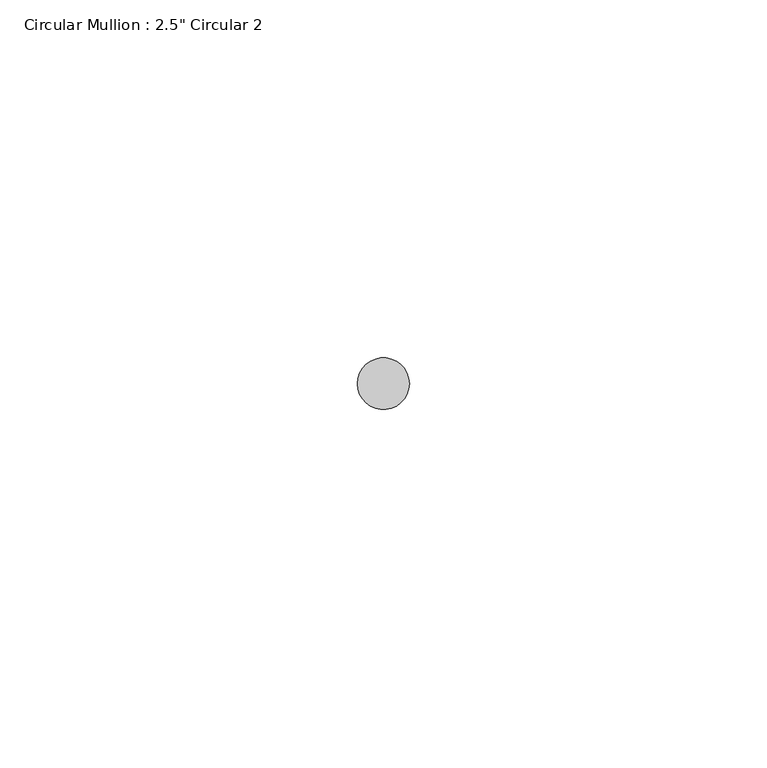
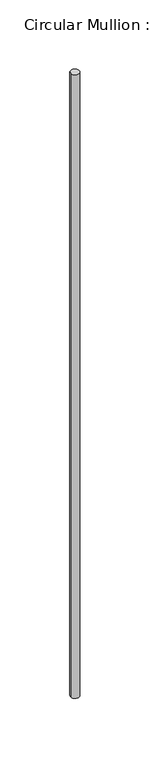
"""IFC4 building model written with IfcOpenShell, lengths in millimetres: member geometry."""

from ifc_helpers import new_model, si_unit, point, frame, frame_2d, origin, place, context, project, spatial, circle_curve, trimmed, segment, composite_curve, outline, extrude, source, transform, mapped, element, save


def member_bd529d22(model_context):
    return source(origin(), model_context, "Body", "SweptSolid", [
        extrude(outline(composite_curve([segment(trimmed(circle_curve(frame_2d((-3.6195, 0.0)), 3.6195), [point((0.0, 0.0))], [point((-7.239, 0.0))], False, "CARTESIAN"), True, "CONTINUOUS"), segment(trimmed(circle_curve(frame_2d((-3.6195, 0.0)), 3.6195), [point((-7.239, 0.0))], [point((0.0, 0.0))], False, "CARTESIAN"), True, "CONTINUOUS")], self_intersect=False)), frame((0.0, 0.0, -558.8), z_axis=(0.0, 0.0, 1.0), x_axis=(1.0, 0.0, 0.0)), (0.0, 0.0, 1.0), 558.8),
    ])


if __name__ == "__main__":
    model = new_model("IFC4")
    model_context = context("Model", 3, world=origin())
    ifc_project = project(units=[si_unit("LENGTHUNIT", "METRE", prefix="MILLI")], contexts=[model_context])
    site = spatial("IfcSite", under=ifc_project)
    building = spatial("IfcBuilding", under=site)
    placement = place(None, origin())
    member_shape = member_bd529d22(model_context)
    element("IfcMember", 1, ObjectType="Circular Mullion : 2.5\" Circular 2", at=placement, inside=building, context=model_context, shape_type="MappedRepresentation", body=[
        mapped(member_shape, transform((0.0, 0.0, 0.0), x_axis=(1.0, 0.0, 0.0), y_axis=(0.0, 1.0, 0.0), z_axis=(0.0, 0.0, 1.0))),
    ])
    save(model, "model.ifc")

# Revit data of these elements
# Type "Circular Mullion : 2.5\" Circular 2"
#   built-in parameter 1007350 = 0.011875 (stored number, unit not read)
# Element 1 (IfcMember, "Circular Mullion : 2.5\" Circular 2")
#   Materials on its faces: "Aluminum"
# Materials
#   "Aluminum": class "Metal", colour RGB 247 247 247, transparency 0, Description = "Aluminum 6061", Cost = 0
